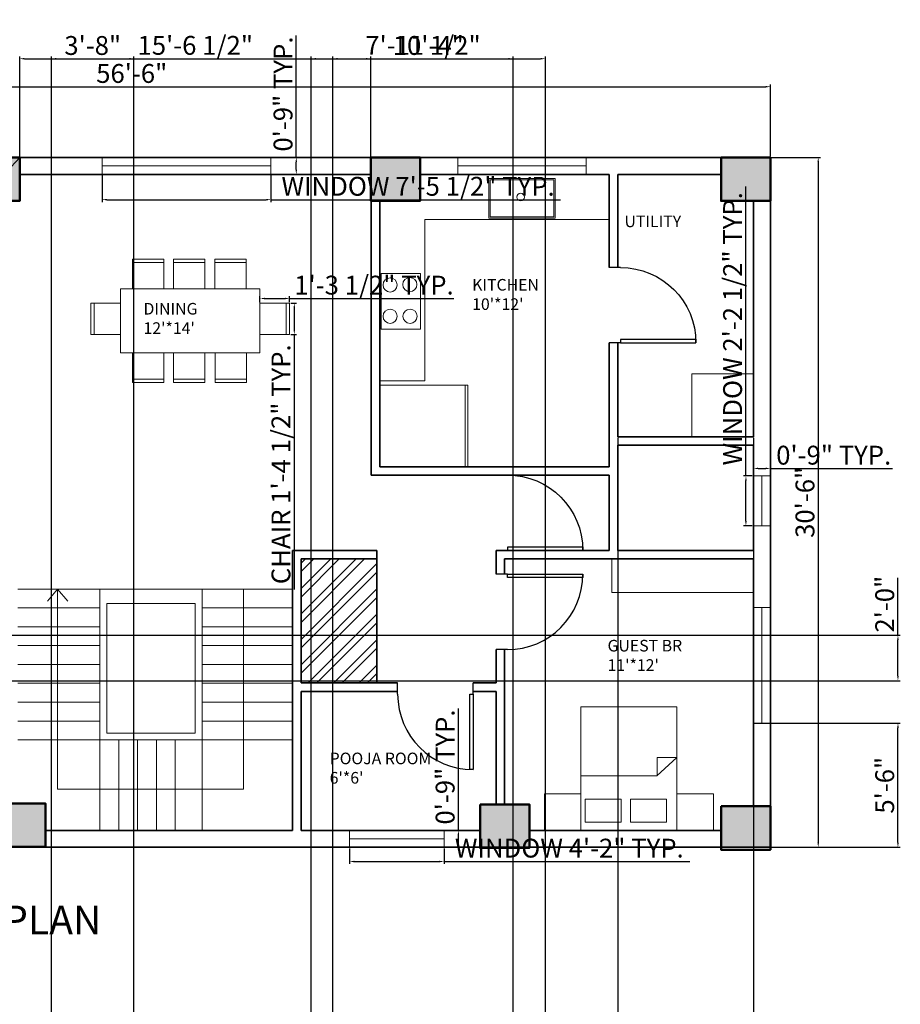
# Model space of a CAD drawing. Units: inches. Extents: x 1964 to 3462, y 1879 to 2909.
# Tile 4 of 4: x 2982 to 3450, y 2387 to 2909. Entities that reach past the tile are written whole.
import ezdxf

# ---------------------------------------------------------------- set-up
doc = ezdxf.new("R2010")
doc.units = ezdxf.units.IN
for name, color, linetype, lineweight in [('A-ANNO-DIMS', 2, 'Continuous', 18), ('A-ANNO-TEXT', 7, 'Continuous', 35), ('A-AREA-IDEN', 7, 'Continuous', 18), ('A-COLS', 1, 'Continuous', 50), ('A-COLS-PATT', 252, 'Continuous', 13), ('A-DOOR', 4, 'Continuous', 25), ('A-EQPM', 9, 'Continuous', 18), ('A-FLOR-CASE', 9, 'Continuous', 18), ('A-FLOR-FIXT', 4, 'Continuous', 18), ('A-FLOR-OPEN', 8, 'Continuous', 13), ('A-FLOR-PATT', 252, 'Continuous', 13), ('A-FLOR-STRS', 3, 'Continuous', 18), ('A-FURN', 8, 'Continuous', 18), ('A-GLAZ', 4, 'Continuous', 18), ('A-WALL', 7, 'Continuous', 35)]:
    doc.layers.add(name, color=color, linetype=linetype, lineweight=lineweight)
doc.styles.get("Standard").update_dxf_attribs({"font": 'arial.ttf'})
doc.dimstyles.new('ISO-25', dxfattribs={"dimtxt": 10, "dimasz": 2.5, "dimexe": 1.25, "dimexo": 0.625, "dimtad": 1, "dimdec": 0, "dimlunit": 4, "dimtxsty": 'Standard', "dimcen": 2.5, "dimadec": 0, "dimazin": 0, "dimtfac": 1, "dimtdec": 0, "dimtmove": 0, "dimatfit": 3, "dimfxl": 1, "dimarcsym": 0})

# ---------------------------------------------------------------- blocks, each defined once
blk = doc.blocks.new('*U2')
for p, q in [((0, 0), (0, -6)), ((40, 0), (40, -6))]:
    blk.add_line(p, q)
blk.add_lwpolyline([(0, 0), (0, 40), (1.75, 40), (1.75, 0)], close=True)
blk.add_arc((0, 0), 40, 0, 90)
blk = doc.blocks.new('*D9')
at = {"layer": 'A-ANNO-DIMS', "color": 0, "lineweight": -2, "transparency": 16777216}
for p, q in [((2702.98, 2836.98), (2702.98, 2875.1)), ((2705.48, 2873.85), (3378.17, 2873.85)), ((3380.67, 2836.98), (3380.67, 2875.1))]:
    blk.add_line(p, q, dxfattribs=at)
at = {"layer": 'A-ANNO-DIMS', "color": 0, "lineweight": 100, "transparency": 16777216}
for points in [[(2705.48, 2874.26), (2705.48, 2873.43), (2702.98, 2873.85)], [(3378.17, 2874.26), (3378.17, 2873.43), (3380.67, 2873.85)]]:
    blk.add_solid(points, dxfattribs=at)
at = {"layer": 'Defpoints', "color": 0, "lineweight": 100, "transparency": 16777216}
for p in [(3380.67, 2873.85), (2702.98, 2836.36), (3380.67, 2836.36)]:
    blk.add_point(p, dxfattribs=at)
at = {"layer": 'A-ANNO-DIMS', "color": 0, "transparency": 16777216, "insert": (3041.82, 2879.58), "char_height": 10, "attachment_point": 5}
blk.add_mtext('56\'-6"', dxfattribs=at)
blk = doc.blocks.new('*D10')
at = {"layer": 'A-ANNO-DIMS', "color": 0, "lineweight": -2, "transparency": 16777216}
for p, q in [((3381.3, 2836.36), (3407.29, 2836.36)), ((3406.04, 2833.86), (3406.04, 2472.86)), ((3381.3, 2470.36), (3407.29, 2470.36))]:
    blk.add_line(p, q, dxfattribs=at)
at = {"layer": 'A-ANNO-DIMS', "color": 0, "lineweight": 100, "transparency": 16777216}
for points in [[(3405.63, 2833.86), (3406.46, 2833.86), (3406.04, 2836.36)], [(3405.63, 2472.86), (3406.46, 2472.86), (3406.04, 2470.36)]]:
    blk.add_solid(points, dxfattribs=at)
at = {"layer": 'Defpoints', "color": 0, "lineweight": 100, "transparency": 16777216}
for p in [(3380.67, 2836.36), (3380.67, 2470.36), (3406.04, 2470.36)]:
    blk.add_point(p, dxfattribs=at)
at = {"layer": 'A-ANNO-DIMS', "color": 0, "transparency": 16777216, "insert": (3400.31, 2653.36), "char_height": 10, "attachment_point": 5, "rotation": 90}
blk.add_mtext('30\'-6"', dxfattribs=at)
blk = doc.blocks.new('COL-RECT-26x23')
blk.add_lwpolyline([(0, 23.08), (26.15, 23.08), (26.15, 0), (0, 0)], close=True)
blk = doc.blocks.new('BED-DOUBLE-WITH-NIGHTSTANDS')
for p, q in [((59.67, 28.98), (70.38, 38.71)), ((70.38, 38.71), (59.8, 38.58)), ((59.8, 38.58), (59.8, 29.09)), ((19.34, 28.98), (59.67, 28.98))]:
    blk.add_line(p, q)
for points in [[(19.34, 0), (70.38, 0), (70.38, 65.5), (19.34, 65.5)], [(19.34, 0), (0, 0), (0, 19.34), (19.34, 19.34)], [(21.67, 4.3), (40.69, 4.3), (40.69, 16.59), (21.67, 16.59)], [(45.74, 4.3), (64.76, 4.3), (64.76, 16.59), (45.74, 16.59)], [(89.72, 0), (70.38, 0), (70.38, 19.34), (89.72, 19.34)]]:
    blk.add_lwpolyline(points, close=True)
blk = doc.blocks.new('CHAIR-DINING')
blk.add_line((0, 13.93), (16.58, 13.93))
blk.add_lwpolyline([(0, 0), (16.58, 0), (16.58, 15.73), (0, 15.73)], close=True)
blk = doc.blocks.new('STAIR-RETURN-RESIDENTIAL')
for p, q in [((0, 128), (145.76, 128)), ((21.08, 128), (15.66, 121.5)), ((21.08, 21.87), (21.08, 128)), ((21.08, 128), (26.5, 121.5)), ((43.5, 124.05), (43.5, 128)), ((97.76, 128), (97.76, 118)), ((119.78, 128), (119.78, 21.87)), ((43.5, 48), (43.5, 124.05)), ((47.14, 51.64), (47.14, 120.41)), ((47.14, 120.41), (94.12, 120.41)), ((94.12, 51.64), (94.12, 120.41)), ((97.76, 48), (97.76, 124.05)), ((0, 118), (43.5, 118)), ((97.76, 118), (145.76, 118)), ((0, 108), (43.5, 108)), ((97.76, 108), (145.76, 108)), ((0, 98), (43.5, 98)), ((97.76, 98), (145.76, 98)), ((0, 88), (43.5, 88)), ((97.76, 88), (145.76, 88)), ((0, 78), (43.5, 78)), ((97.76, 78), (145.76, 78)), ((0, 68), (43.5, 68)), ((97.76, 68), (145.76, 68)), ((0, 58), (43.5, 58)), ((97.76, 58), (145.76, 58)), ((0, 48), (145.76, 48)), ((97.76, 48), (43.5, 48)), ((43.5, 48), (43.5, 0)), ((94.12, 51.64), (47.14, 51.64)), ((53.5, 48), (53.5, 0)), ((63.5, 48), (63.5, 0)), ((73.5, 48), (73.5, 0)), ((83.5, 48), (83.5, 0)), ((97.76, 50.18), (97.76, 0)), ((119.78, 21.87), (21.08, 21.87))]:
    blk.add_line(p, q)
blk = doc.blocks.new('WIN-50IN')
blk.add_line((0, 4.5), (50.22, 4.5))
blk.add_lwpolyline([(0, 9), (50.22, 9), (50.22, 0), (0, 0)], close=True)
blk = doc.blocks.new('WIN-61IN')
blk.add_line((4.5, 61.35), (4.5, 0))
blk.add_lwpolyline([(0, 61.35), (9, 61.35), (9, 0), (0, 0)], close=True)
blk = doc.blocks.new('WIN-27IN')
blk.add_line((4.5, 26.51), (4.5, 0))
blk.add_lwpolyline([(0, 0), (9, 0), (9, 26.51), (0, 26.51)], close=True)
blk = doc.blocks.new('WIN-90IN')
blk.add_line((0, 4.5), (89.57, 4.5))
blk.add_lwpolyline([(0, 9), (89.57, 9), (89.57, 0), (0, 0)], close=True)
blk = doc.blocks.new('*D27')
at = {"layer": 'A-ANNO-DIMS', "color": 0, "lineweight": -2, "transparency": 16777216}
for p, q in [((3126.2, 2759.01), (3129.32, 2759.01)), ((3128.07, 2756.51), (3128.07, 2744.93)), ((3126.2, 2742.43), (3129.32, 2742.43)), ((3128.07, 2742.43), (3128.07, 2607.19))]:
    blk.add_line(p, q, dxfattribs=at)
at = {"layer": 'A-ANNO-DIMS', "color": 0, "lineweight": 100, "transparency": 16777216}
for points in [[(3127.65, 2756.51), (3128.48, 2756.51), (3128.07, 2759.01)], [(3127.65, 2744.93), (3128.48, 2744.93), (3128.07, 2742.43)]]:
    blk.add_solid(points, dxfattribs=at)
at = {"layer": 'Defpoints', "color": 0, "lineweight": 100, "transparency": 16777216}
for p in [(3125.58, 2759.01), (3125.58, 2742.43), (3128.07, 2742.43)]:
    blk.add_point(p, dxfattribs=at)
at = {"layer": 'A-ANNO-DIMS', "color": 0, "transparency": 16777216, "insert": (3122.27, 2673.56), "char_height": 10, "attachment_point": 5, "rotation": 90}
blk.add_mtext('CHAIR 1\'-4 1/2" TYP.', dxfattribs=at)
blk = doc.blocks.new('*D28')
at = {"layer": 'A-ANNO-DIMS', "color": 0, "lineweight": -2, "transparency": 16777216}
for p, q in [((3109.85, 2759.63), (3109.85, 2762.74)), ((3112.35, 2761.49), (3123.08, 2761.49)), ((3125.58, 2759.63), (3125.58, 2762.74)), ((3125.58, 2761.49), (3212.64, 2761.49))]:
    blk.add_line(p, q, dxfattribs=at)
at = {"layer": 'A-ANNO-DIMS', "color": 0, "lineweight": 100, "transparency": 16777216}
for points in [[(3112.35, 2761.91), (3112.35, 2761.08), (3109.85, 2761.49)], [(3123.08, 2761.91), (3123.08, 2761.08), (3125.58, 2761.49)]]:
    blk.add_solid(points, dxfattribs=at)
at = {"layer": 'Defpoints', "color": 0, "lineweight": 100, "transparency": 16777216}
for p in [(3109.85, 2759.01), (3125.58, 2761.49), (3125.58, 2759.01)]:
    blk.add_point(p, dxfattribs=at)
at = {"layer": 'A-ANNO-DIMS', "color": 0, "transparency": 16777216, "insert": (3170.36, 2767.29), "char_height": 10, "attachment_point": 5}
blk.add_mtext('1\'-3 1/2" TYP.', dxfattribs=at)
blk = doc.blocks.new('*D35')
at = {"layer": 'A-ANNO-DIMS', "color": 0, "lineweight": -2, "transparency": 16777216}
for p, q in [((3157.37, 2469.73), (3157.37, 2461.58)), ((3207.59, 2469.73), (3207.59, 2461.58)), ((3159.87, 2462.83), (3205.09, 2462.83)), ((3207.59, 2462.83), (3337.88, 2462.83))]:
    blk.add_line(p, q, dxfattribs=at)
at = {"layer": 'A-ANNO-DIMS', "color": 0, "lineweight": 100, "transparency": 16777216}
for points in [[(3159.87, 2463.24), (3159.87, 2462.41), (3157.37, 2462.83)], [(3205.09, 2463.24), (3205.09, 2462.41), (3207.59, 2462.83)]]:
    blk.add_solid(points, dxfattribs=at)
at = {"layer": 'Defpoints', "color": 0, "lineweight": 100, "transparency": 16777216}
for p in [(3157.37, 2470.36), (3207.59, 2470.36), (3207.59, 2462.83)]:
    blk.add_point(p, dxfattribs=at)
at = {"layer": 'A-ANNO-DIMS', "color": 0, "transparency": 16777216, "insert": (3273.98, 2468.63), "char_height": 10, "attachment_point": 5}
blk.add_mtext('WINDOW 4\'-2" TYP.', dxfattribs=at)
blk = doc.blocks.new('*D36')
at = {"layer": 'A-ANNO-DIMS', "color": 0, "lineweight": -2, "transparency": 16777216}
for p, q in [((3215.12, 2479.36), (3215.12, 2544.06)), ((3208.21, 2479.36), (3216.37, 2479.36)), ((3215.12, 2472.86), (3215.12, 2476.86)), ((3208.21, 2470.36), (3216.37, 2470.36))]:
    blk.add_line(p, q, dxfattribs=at)
at = {"layer": 'A-ANNO-DIMS', "color": 0, "lineweight": 100, "transparency": 16777216}
for points in [[(3214.7, 2476.86), (3215.54, 2476.86), (3215.12, 2479.36)], [(3214.7, 2472.86), (3215.54, 2472.86), (3215.12, 2470.36)]]:
    blk.add_solid(points, dxfattribs=at)
at = {"layer": 'Defpoints', "color": 0, "lineweight": 100, "transparency": 16777216}
for p in [(3207.59, 2479.36), (3215.12, 2479.36), (3207.59, 2470.36)]:
    blk.add_point(p, dxfattribs=at)
at = {"layer": 'A-ANNO-DIMS', "color": 0, "transparency": 16777216, "insert": (3209.39, 2512.96), "char_height": 10, "attachment_point": 5, "rotation": 90}
blk.add_mtext('0\'-9" TYP.', dxfattribs=at)
blk = doc.blocks.new('*D39')
at = {"layer": 'A-ANNO-DIMS', "color": 0, "lineweight": -2, "transparency": 16777216}
for p, q in [((3367.7, 2667.38), (3367.7, 2820.98)), ((3371.05, 2667.38), (3366.45, 2667.38)), ((3367.7, 2643.38), (3367.7, 2664.88)), ((3371.05, 2640.88), (3366.45, 2640.88))]:
    blk.add_line(p, q, dxfattribs=at)
at = {"layer": 'A-ANNO-DIMS', "color": 0, "lineweight": 100, "transparency": 16777216}
for points in [[(3367.28, 2664.88), (3368.11, 2664.88), (3367.7, 2667.38)], [(3367.28, 2643.38), (3368.11, 2643.38), (3367.7, 2640.88)]]:
    blk.add_solid(points, dxfattribs=at)
at = {"layer": 'Defpoints', "color": 0, "lineweight": 100, "transparency": 16777216}
for p in [(3367.7, 2667.38), (3371.67, 2667.38), (3371.67, 2640.88)]:
    blk.add_point(p, dxfattribs=at)
at = {"layer": 'A-ANNO-DIMS', "color": 0, "transparency": 16777216, "insert": (3361.9, 2745.43), "char_height": 10, "attachment_point": 5, "rotation": 90}
blk.add_mtext('WINDOW 2\'-2 1/2" TYP.', dxfattribs=at)
blk = doc.blocks.new('*D40')
at = {"layer": 'A-ANNO-DIMS', "color": 0, "lineweight": -2, "transparency": 16777216}
for p, q in [((3371.67, 2668.01), (3371.67, 2672.61)), ((3374.17, 2671.36), (3378.17, 2671.36)), ((3380.67, 2668.01), (3380.67, 2672.61)), ((3380.67, 2671.36), (3445.38, 2671.36))]:
    blk.add_line(p, q, dxfattribs=at)
at = {"layer": 'A-ANNO-DIMS', "color": 0, "lineweight": 100, "transparency": 16777216}
for points in [[(3374.17, 2671.78), (3374.17, 2670.94), (3371.67, 2671.36)], [(3378.17, 2671.78), (3378.17, 2670.94), (3380.67, 2671.36)]]:
    blk.add_solid(points, dxfattribs=at)
at = {"layer": 'Defpoints', "color": 0, "lineweight": 100, "transparency": 16777216}
for p in [(3380.67, 2671.36), (3371.67, 2667.38), (3380.67, 2667.38)]:
    blk.add_point(p, dxfattribs=at)
at = {"layer": 'A-ANNO-DIMS', "color": 0, "transparency": 16777216, "insert": (3414.27, 2677.09), "char_height": 10, "attachment_point": 5}
blk.add_mtext('0\'-9" TYP.', dxfattribs=at)
blk = doc.blocks.new('*D41')
at = {"layer": 'A-ANNO-DIMS', "color": 0, "lineweight": -2, "transparency": 16777216}
for p, q in [((3026.12, 2826.73), (3026.12, 2812.67)), ((3115.69, 2826.73), (3115.69, 2812.67)), ((3028.62, 2813.92), (3113.19, 2813.92)), ((3115.69, 2813.92), (3269.28, 2813.92))]:
    blk.add_line(p, q, dxfattribs=at)
at = {"layer": 'A-ANNO-DIMS', "color": 0, "lineweight": 100, "transparency": 16777216}
for points in [[(3028.62, 2814.34), (3028.62, 2813.51), (3026.12, 2813.92)], [(3113.19, 2814.34), (3113.19, 2813.51), (3115.69, 2813.92)]]:
    blk.add_solid(points, dxfattribs=at)
at = {"layer": 'Defpoints', "color": 0, "lineweight": 100, "transparency": 16777216}
for p in [(3026.12, 2827.36), (3115.69, 2827.36), (3115.69, 2813.92)]:
    blk.add_point(p, dxfattribs=at)
at = {"layer": 'A-ANNO-DIMS', "color": 0, "transparency": 16777216, "insert": (3193.74, 2819.72), "char_height": 10, "attachment_point": 5}
blk.add_mtext('WINDOW 7\'-5 1/2" TYP.', dxfattribs=at)
blk = doc.blocks.new('*D42')
at = {"layer": 'A-ANNO-DIMS', "color": 0, "lineweight": -2, "transparency": 16777216}
for p, q in [((3129.13, 2836.36), (3129.13, 2901.06)), ((3116.32, 2836.36), (3130.38, 2836.36)), ((3129.13, 2829.86), (3129.13, 2833.86)), ((3116.32, 2827.36), (3130.38, 2827.36))]:
    blk.add_line(p, q, dxfattribs=at)
at = {"layer": 'A-ANNO-DIMS', "color": 0, "lineweight": 100, "transparency": 16777216}
for points in [[(3128.71, 2833.86), (3129.54, 2833.86), (3129.13, 2836.36)], [(3128.71, 2829.86), (3129.54, 2829.86), (3129.13, 2827.36)]]:
    blk.add_solid(points, dxfattribs=at)
at = {"layer": 'Defpoints', "color": 0, "lineweight": 100, "transparency": 16777216}
for p in [(3115.69, 2836.36), (3129.13, 2836.36), (3115.69, 2827.36)]:
    blk.add_point(p, dxfattribs=at)
at = {"layer": 'A-ANNO-DIMS', "color": 0, "transparency": 16777216, "insert": (3123.39, 2869.96), "char_height": 10, "attachment_point": 5, "rotation": 90}
blk.add_mtext('0\'-9" TYP.', dxfattribs=at)
blk = doc.blocks.new('*D55')
at = {"layer": 'A-ANNO-DIMS', "color": 0, "lineweight": -2, "transparency": 16777216}
for p, q in [((2982.37, 2813.9), (2982.37, 2889.94)), ((2984.87, 2888.69), (3166.19, 2888.69)), ((3168.69, 2813.9), (3168.69, 2889.94))]:
    blk.add_line(p, q, dxfattribs=at)
at = {"layer": 'A-ANNO-DIMS', "color": 0, "lineweight": 100, "transparency": 16777216}
for points in [[(2984.87, 2889.1), (2984.87, 2888.27), (2982.37, 2888.69)], [(3166.19, 2889.1), (3166.19, 2888.27), (3168.69, 2888.69)]]:
    blk.add_solid(points, dxfattribs=at)
at = {"layer": 'Defpoints', "color": 0, "lineweight": 100, "transparency": 16777216}
for p in [(3168.69, 2888.69), (2982.37, 2813.28), (3168.69, 2813.28)]:
    blk.add_point(p, dxfattribs=at)
at = {"layer": 'A-ANNO-DIMS', "color": 0, "transparency": 16777216, "insert": (3075.53, 2894.48), "char_height": 10, "attachment_point": 5}
blk.add_mtext('15\'-6 1/2"', dxfattribs=at)
blk = doc.blocks.new('*D56')
at = {"layer": 'A-ANNO-DIMS', "color": 0, "lineweight": -2, "transparency": 16777216}
for p, q in [((3299.67, 2687.56), (3299.67, 1887.22)), ((3371.67, 2687.56), (3371.67, 1887.22)), ((3302.17, 1888.47), (3369.17, 1888.47))]:
    blk.add_line(p, q, dxfattribs=at)
at = {"layer": 'A-ANNO-DIMS', "color": 0, "lineweight": 100, "transparency": 16777216}
for points in [[(3302.17, 1888.89), (3302.17, 1888.06), (3299.67, 1888.47)], [(3369.17, 1888.89), (3369.17, 1888.06), (3371.67, 1888.47)]]:
    blk.add_solid(points, dxfattribs=at)
at = {"layer": 'Defpoints', "color": 0, "lineweight": 100, "transparency": 16777216}
for p in [(3299.67, 2688.18), (3371.67, 2688.18), (3371.67, 1888.47)]:
    blk.add_point(p, dxfattribs=at)
at = {"layer": 'A-ANNO-DIMS', "color": 0, "transparency": 16777216, "insert": (3335.67, 1894.2), "char_height": 10, "attachment_point": 5}
blk.add_mtext('6\'-0"', dxfattribs=at)
blk = doc.blocks.new('*D60')
at = {"layer": 'A-ANNO-DIMS', "color": 0, "lineweight": -2, "transparency": 16777216}
for p, q in [((3448.35, 2582.86), (3448.35, 2613.36)), ((2815.81, 2582.86), (3449.6, 2582.86)), ((3448.35, 2561.25), (3448.35, 2580.36)), ((2815.81, 2558.75), (3449.6, 2558.75))]:
    blk.add_line(p, q, dxfattribs=at)
at = {"layer": 'A-ANNO-DIMS', "color": 0, "lineweight": 100, "transparency": 16777216}
for points in [[(3447.94, 2580.36), (3448.77, 2580.36), (3448.35, 2582.86)], [(3447.94, 2561.25), (3448.77, 2561.25), (3448.35, 2558.75)]]:
    blk.add_solid(points, dxfattribs=at)
at = {"layer": 'Defpoints', "color": 0, "lineweight": 100, "transparency": 16777216}
for p in [(2815.18, 2582.86), (3448.35, 2582.86), (2815.18, 2558.75)]:
    blk.add_point(p, dxfattribs=at)
at = {"layer": 'A-ANNO-DIMS', "color": 0, "transparency": 16777216, "insert": (3442.62, 2599.36), "char_height": 10, "attachment_point": 5, "rotation": 90}
blk.add_mtext('2\'-0"', dxfattribs=at)
blk = doc.blocks.new('*D61')
at = {"layer": 'A-ANNO-DIMS', "color": 0, "lineweight": -2, "transparency": 16777216}
for p, q in [((3372.3, 2536.22), (3449.6, 2536.22)), ((3448.35, 2472.86), (3448.35, 2533.72)), ((3381.3, 2470.36), (3449.6, 2470.36))]:
    blk.add_line(p, q, dxfattribs=at)
at = {"layer": 'A-ANNO-DIMS', "color": 0, "lineweight": 100, "transparency": 16777216}
for points in [[(3447.94, 2533.72), (3448.77, 2533.72), (3448.35, 2536.22)], [(3447.94, 2472.86), (3448.77, 2472.86), (3448.35, 2470.36)]]:
    blk.add_solid(points, dxfattribs=at)
at = {"layer": 'Defpoints', "color": 0, "lineweight": 100, "transparency": 16777216}
for p in [(3371.67, 2536.22), (3448.35, 2536.22), (3380.67, 2470.36)]:
    blk.add_point(p, dxfattribs=at)
at = {"layer": 'A-ANNO-DIMS', "color": 0, "transparency": 16777216, "insert": (3442.62, 2503.29), "char_height": 10, "attachment_point": 5, "rotation": 90}
blk.add_mtext('5\'-6"', dxfattribs=at)
blk = doc.blocks.new('*D65')
at = {"layer": 'A-ANNO-DIMS', "color": 0, "lineweight": -2, "transparency": 16777216}
for p, q in [((3137.07, 2298.2), (3137.07, 2889.94)), ((3139.57, 2888.69), (3258.77, 2888.69)), ((3261.27, 2298.2), (3261.27, 2889.94))]:
    blk.add_line(p, q, dxfattribs=at)
at = {"layer": 'A-ANNO-DIMS', "color": 0, "lineweight": 100, "transparency": 16777216}
for points in [[(3139.57, 2889.1), (3139.57, 2888.27), (3137.07, 2888.69)], [(3258.77, 2889.1), (3258.77, 2888.27), (3261.27, 2888.69)]]:
    blk.add_solid(points, dxfattribs=at)
at = {"layer": 'Defpoints', "color": 0, "lineweight": 100, "transparency": 16777216}
for p in [(3261.27, 2888.69), (3137.07, 2297.57), (3261.27, 2297.57)]:
    blk.add_point(p, dxfattribs=at)
at = {"layer": 'A-ANNO-DIMS', "color": 0, "transparency": 16777216, "insert": (3199.17, 2894.42), "char_height": 10, "attachment_point": 5}
blk.add_mtext('10\'-4"', dxfattribs=at)
blk = doc.blocks.new('*D67')
at = {"layer": 'A-ANNO-DIMS', "color": 0, "lineweight": -2, "transparency": 16777216}
for p, q in [((3148.55, 2033.75), (3148.55, 2889.94)), ((3151.05, 2888.69), (3241.63, 2888.69)), ((3244.13, 2034), (3244.13, 2889.94))]:
    blk.add_line(p, q, dxfattribs=at)
at = {"layer": 'A-ANNO-DIMS', "color": 0, "lineweight": 100, "transparency": 16777216}
for points in [[(3151.05, 2889.1), (3151.05, 2888.27), (3148.55, 2888.69)], [(3241.63, 2889.1), (3241.63, 2888.27), (3244.13, 2888.69)]]:
    blk.add_solid(points, dxfattribs=at)
at = {"layer": 'Defpoints', "color": 0, "lineweight": 100, "transparency": 16777216}
for p in [(3244.13, 2888.69), (3148.55, 2033.12), (3244.13, 2033.37)]:
    blk.add_point(p, dxfattribs=at)
at = {"layer": 'A-ANNO-DIMS', "color": 0, "transparency": 16777216, "insert": (3196.34, 2894.48), "char_height": 10, "attachment_point": 5}
blk.add_mtext('7\'-11 1/2"', dxfattribs=at)
blk = doc.blocks.new('*D68')
at = {"layer": 'A-ANNO-DIMS', "color": 0, "lineweight": -2, "transparency": 16777216}
for p, q in [((2999.25, 2307.2), (2999.25, 2889.94)), ((3001.75, 2888.69), (3040.51, 2888.69)), ((3043.01, 2307.2), (3043.01, 2889.94))]:
    blk.add_line(p, q, dxfattribs=at)
at = {"layer": 'A-ANNO-DIMS', "color": 0, "lineweight": 100, "transparency": 16777216}
for points in [[(3001.75, 2889.1), (3001.75, 2888.27), (2999.25, 2888.69)], [(3040.51, 2889.1), (3040.51, 2888.27), (3043.01, 2888.69)]]:
    blk.add_solid(points, dxfattribs=at)
at = {"layer": 'Defpoints', "color": 0, "lineweight": 100, "transparency": 16777216}
for p in [(3043.01, 2888.69), (2999.25, 2306.57), (3043.01, 2306.57)]:
    blk.add_point(p, dxfattribs=at)
at = {"layer": 'A-ANNO-DIMS', "color": 0, "transparency": 16777216, "insert": (3021.13, 2894.42), "char_height": 10, "attachment_point": 5}
blk.add_mtext('3\'-8"', dxfattribs=at)

msp = doc.modelspace()

# ---------------------------------------------------------------- hatches: boundary and pattern name
at = {"layer": 'A-COLS-PATT'}
h = msp.add_hatch(color=256, dxfattribs=at)
h.dxf.hatch_style = 1
h.paths.add_polyline_path([(3380.67, 2836.36), (3354.52, 2836.36), (3354.52, 2813.28), (3380.67, 2813.28)])
h.paths.add_polyline_path([(3194.85, 2836.36), (3168.69, 2836.36), (3168.69, 2827.36), (3168.91, 2827.36), (3168.91, 2813.28), (3194.85, 2813.28)])
h.paths.add_polyline_path([(2982.37, 2836.36), (2956.21, 2836.36), (2956.21, 2813.28), (2961, 2813.28)])
h.paths.add_polyline_path([(2982.37, 2836.36), (2961, 2813.28), (2981.41, 2813.28), (2982.37, 2813.28)], flags=17)
h.paths.add_polyline_path([(2831.78, 2494.67), (2805.62, 2494.67), (2805.62, 2471.58), (2831.78, 2471.58)])
h.paths.add_polyline_path([(2995.98, 2493.63), (2969.83, 2493.63), (2969.83, 2470.55), (2995.98, 2470.55)])
h.paths.add_polyline_path([(3252.83, 2493.16), (3226.67, 2493.16), (3226.67, 2470.36), (3252.83, 2470.36)])
h.paths.add_polyline_path([(3380.67, 2492.15), (3354.52, 2492.15), (3354.52, 2470.36), (3380.67, 2470.36)])
at = {"layer": 'A-FLOR-PATT'}
h = msp.add_hatch(dxfattribs=at)
h.set_pattern_fill('ANSI32', color=256)
h.set_pattern_definition([(45, (161.698, 257.281), (-6.735192, 6.735192), []), (45, (166.188, 257.281), (-6.735192, 6.735192), [])])
h.paths.add_polyline_path([(3131.67, 2557.57), (3171.89, 2557.57), (3171.89, 2623.36), (3131.67, 2623.36)])
h.paths.add_polyline_path([(3164.38, 2278.1), (3261.27, 2278.1), (3261.27, 2297.57), (3231.68, 2297.57), (3211.73, 2297.57), (3211.73, 2283.49), (3185.58, 2283.49), (3185.58, 2297.57), (3166.29, 2297.57), (3142.29, 2297.57), (3137.07, 2297.57), (3137.07, 2154.78), (3164.38, 2154.78)])
h.paths.add_polyline_path([(2977.34, 2283.49), (2973.1, 2283.49), (2973.1, 2297.57), (2946.77, 2297.57), (2946.77, 2213.49), (2977.34, 2213.49)])
h.paths.add_polyline_path([(3313.48, 2093.57), (3313.48, 2075.7), (3388.55, 2075.7), (3388.55, 2093.57)])
h.paths.add_polyline_path([(3161.01, 2228.59), (3238.21, 2228.59), (3238.21, 2241.28), (3161.01, 2241.28)], flags=24)

# ---------------------------------------------------------------- linework, layer by layer
at = {"layer": 'A-EQPM'}
for points in [[(3174.19, 2774.84), (3195.11, 2774.84), (3195.11, 2745.16), (3174.19, 2745.16)], [(3371.67, 2688.18), (3339, 2688.18), (3339, 2721.57), (3371.67, 2721.57)]]:
    msp.add_lwpolyline(points, close=True, dxfattribs=at)
for centre in [(3178.9, 2768.68), (3189.36, 2768.89), (3178.9, 2752.06), (3189.47, 2752.06)]:
    msp.add_circle(centre, 3.76, dxfattribs=at)
at = {"layer": 'A-FLOR-CASE'}
for p, q in [((3295.17, 2827.36), (3295.17, 2803.36)), ((3197.41, 2717.82), (3197.41, 2803.36)), ((3295.17, 2803.36), (3197.41, 2803.36)), ((3173.41, 2717.82), (3197.41, 2717.82)), ((3218.8, 2672.28), (3218.8, 2715.58))]:
    msp.add_line(p, q, dxfattribs=at)
for points in [[(3173.41, 2672.28), (3220.22, 2672.28), (3220.22, 2715.58), (3173.41, 2715.58)], [(3371.67, 2623.36), (3296.59, 2623.36), (3296.59, 2605.49), (3371.67, 2605.49)]]:
    msp.add_lwpolyline(points, close=True, dxfattribs=at)
at = {"layer": 'A-FLOR-FIXT'}
for points in [[(3231.34, 2804.15), (3266.43, 2804.15), (3266.43, 2825.23), (3231.34, 2825.23)], [(3232.07, 2804.88), (3265.7, 2804.88), (3265.7, 2824.5), (3232.07, 2824.5)]]:
    msp.add_lwpolyline(points, close=True, dxfattribs=at)
msp.add_circle((3248.15, 2815.32), 1.98, dxfattribs=at)
at = {"layer": 'A-FLOR-OPEN'}
msp.add_line((2751.91, 2587.36), (2982.37, 2836.36), dxfattribs=at)
at = {"layer": 'A-FLOR-STRS'}
for q in [(3127.17, 2515.36), (3091.17, 2479.36), (3091.17, 2479.36)]:
    msp.add_line((3127.17, 2479.36), q, dxfattribs=at)
at = {"layer": 'A-FURN'}
msp.add_lwpolyline([(3035.8, 2766.67), (3109.85, 2766.67), (3109.85, 2732.61), (3035.8, 2732.61)], close=True, dxfattribs=at)
at = {"layer": 'A-GLAZ'}
msp.add_line((3214.8, 2831.86), (3282.98, 2831.86), dxfattribs=at)
msp.add_lwpolyline([(3214.8, 2836.36), (3282.98, 2836.36), (3282.98, 2827.36), (3214.8, 2827.36)], close=True, dxfattribs=at)
at = {"layer": 'A-WALL'}
for p, q in [((3380.67, 2836.36), (3380.67, 2470.36)), ((2982.37, 2827.36), (3125.41, 2827.36)), ((3125.41, 2827.36), (3149.41, 2827.36)), ((3149.41, 2827.36), (3168.91, 2827.36)), ((3168.91, 2827.36), (3168.91, 2667.78)), ((3295.17, 2827.36), (3295.17, 2777.95)), ((3354.52, 2827.36), (3299.67, 2827.36)), ((3299.67, 2827.36), (3299.67, 2777.95)), ((3173.41, 2813.28), (3173.41, 2672.28)), ((3295.17, 2737.95), (3295.17, 2707.36)), ((3299.67, 2737.95), (3299.67, 2707.36)), ((3295.17, 2707.36), (3295.17, 2672.28)), ((3299.67, 2707.36), (3299.67, 2688.18)), ((3299.67, 2688.18), (3371.67, 2688.18)), ((3299.67, 2683.68), (3371.67, 2683.68)), ((3299.67, 2683.68), (3299.67, 2627.86)), ((3355.57, 2683.68), (3371.67, 2683.68)), ((3295.17, 2672.28), (3173.41, 2672.28)), ((3295.17, 2667.78), (3168.91, 2667.78)), ((3295.17, 2667.78), (3295.17, 2627.86)), ((3127.17, 2479.36), (3127.17, 2627.86)), ((3127.17, 2627.86), (3171.89, 2627.86)), ((3171.89, 2557.57), (3171.89, 2627.86)), ((3235.17, 2623.36), (3235.17, 2627.86)), ((3235.17, 2627.86), (3246.85, 2627.86)), ((3295.17, 2627.86), (3235.17, 2627.86)), ((3371.67, 2627.86), (3299.67, 2627.86)), ((3131.67, 2623.36), (3171.89, 2623.36)), ((3131.67, 2557.57), (3131.67, 2623.36)), ((3235.17, 2623.36), (3235.17, 2615.22)), ((3371.67, 2623.36), (3239.67, 2623.36)), ((3239.67, 2623.36), (3239.67, 2615.22)), ((3239.67, 2623.36), (3246.85, 2623.36)), ((3371.67, 2492.15), (3371.67, 2623.36)), ((3235.17, 2575.22), (3235.17, 2557.57)), ((3239.67, 2575.22), (3239.67, 2493.16)), ((3131.67, 2557.57), (3182.9, 2557.57)), ((3222.9, 2557.57), (3235.17, 2557.57)), ((3131.67, 2479.36), (3131.67, 2553.07)), ((3131.67, 2553.07), (3182.9, 2553.07)), ((3222.9, 2553.07), (3235.17, 2553.07)), ((3235.17, 2553.07), (3235.17, 2493.16)), ((3163.17, 2479.36), (3131.67, 2479.36)), ((3226.67, 2479.36), (3163.17, 2479.36))]:
    msp.add_line(p, q, dxfattribs=at)
for points in [[(2751.91, 2633.6), (2751.91, 2836.36), (3380.67, 2836.36), (3380.67, 2470.36), (2751.91, 2470.36)], [(3380.67, 2674.12), (3380.67, 2836.36), (2841.75, 2836.36)], [(2982.37, 2827.36), (3168.91, 2827.36)], [(3194.85, 2827.36), (3295.17, 2827.36)], [(3299.67, 2827.36), (3354.52, 2827.36)], [(3371.67, 2813.28), (3371.67, 2688.18)], [(3371.67, 2683.68), (3371.67, 2627.86)], [(2841.75, 2470.36), (3380.67, 2470.36), (3380.67, 2634.12)], [(3371.67, 2623.36), (3371.67, 2492.15)], [(3127.17, 2479.36), (2995.98, 2479.36)], [(3226.67, 2479.36), (3131.67, 2479.36)], [(3354.52, 2479.36), (3252.83, 2479.36)]]:
    msp.add_lwpolyline(points, dxfattribs=at)

# ---------------------------------------------------------------- block references
at = {"layer": 'A-COLS'}
for p in [(2956.21, 2813.28), (3168.69, 2813.28), (3354.52, 2813.28), (2969.83, 2470.55), (3226.67, 2470.08), (3354.52, 2469.06)]:
    msp.add_blockref('COL-RECT-26x23', p, dxfattribs=at)
at = {"layer": 'A-DOOR', "xscale": -1, "rotation": 270}
for p in [(3301.17, 2737.95), (3241.17, 2627.86)]:
    msp.add_blockref('*U2', p, dxfattribs=at)
at = {"layer": 'A-DOOR'}
for p, rotation in [((3241.17, 2615.22), 270), ((3222.9, 2551.57), 180)]:
    msp.add_blockref('*U2', p, dxfattribs=dict(at, rotation=rotation))
at = {"layer": 'A-FLOR-STRS'}
msp.add_blockref('STAIR-RETURN-RESIDENTIAL', (2981.41, 2479.36), dxfattribs=at)
at = {"layer": 'A-FURN'}
for name, p in [('CHAIR-DINING', (3042.19, 2766.67)), ('CHAIR-DINING', (3063.95, 2766.67)), ('CHAIR-DINING', (3085.97, 2766.67)), ('BED-DOUBLE-WITH-NIGHTSTANDS', (3260.74, 2479.36))]:
    msp.add_blockref(name, p, dxfattribs=at)
at = {"layer": 'A-FURN', "extrusion": (0, 0, -1), "zscale": -1}
for p, rotation in [((-3035.8, 2759.01), 269.9999999999971), ((-3042.3, 2732.61), 180), ((-3064.05, 2732.61), 180), ((-3086.08, 2732.61), 180)]:
    msp.add_blockref('CHAIR-DINING', p, dxfattribs=dict(at, rotation=rotation))
at = {"layer": 'A-FURN', "rotation": 269.9999999999971}
msp.add_blockref('CHAIR-DINING', (3109.85, 2759.01), dxfattribs=at)
at = {"layer": 'A-GLAZ'}
for name, p in [('WIN-90IN', (3026.12, 2827.36)), ('WIN-27IN', (3371.67, 2640.88)), ('WIN-61IN', (3371.67, 2536.22)), ('WIN-50IN', (3157.37, 2470.36))]:
    msp.add_blockref(name, p, dxfattribs=at)

# ---------------------------------------------------------------- texts
at = {"layer": 'A-ANNO-TEXT', "insert": (2708.78, 2439.45), "char_height": 15.2607, "attachment_point": 1}
msp.add_mtext_dynamic_manual_height_columns('FIRST RESIDENTIAL FLOOR PLAN', width=480.7827, gutter_width=76.3, heights=[0], dxfattribs=at)
at = {"layer": 'A-AREA-IDEN', "char_height": 6.161, "attachment_point": 1}
for s, insert in [('UTILITY', (3303.25, 2805.5)), ("KITCHEN\\P10'*12'", (3222.43, 2771.85)), ("DINING\\P12'*14'", (3048.05, 2759.14)), ("GUEST BR\\P11'*12'", (3294.27, 2580.41)), ("POOJA ROOM\\P6'*6'", (3146.84, 2520.59))]:
    msp.add_mtext_dynamic_manual_height_columns(s, width=194.1034, gutter_width=30.81, heights=[0], dxfattribs=dict(at, insert=insert))

# ---------------------------------------------------------------- dimensions: what is measured, and where the dimension line sits
at = {"layer": 'A-ANNO-DIMS'}
for base, p1, p2, override, picture, middle in [((3168.69, 2888.69), (2982.37, 2813.28), (3168.69, 2813.28), {"dimdec": 1, "dimlfac": 1, "dimrnd": 0, "dimzin": 1, "dimdsep": 46, "dimlunit": 4, "dimfrac": 2}, '*D55', (3075.53, 2894.48)), ((3244.13, 2888.69), (3148.55, 2033.12), (3244.13, 2033.37), {"dimdec": 1, "dimlfac": 1, "dimrnd": 0, "dimzin": 1, "dimdsep": 46, "dimlunit": 4, "dimfrac": 2}, '*D67', (3196.34, 2894.48)), ((3043.01, 2888.69), (2999.25, 2306.57), (3043.01, 2306.57), {"dimdec": 1, "dimlfac": 1, "dimrnd": 0, "dimzin": 1, "dimdsep": 46, "dimlunit": 4, "dimfrac": 2}, '*D68', (3021.13, 2894.42)), ((3261.27, 2888.69), (3137.07, 2297.57), (3261.27, 2297.57), {"dimdec": 1, "dimlfac": 1, "dimrnd": 0, "dimzin": 1, "dimdsep": 46, "dimlunit": 4, "dimfrac": 2}, '*D65', (3199.17, 2894.42)), ((3380.67, 2873.85), (2702.98, 2836.36), (3380.67, 2836.36), {"dimclrd": 0, "dimclre": 0, "dimclrt": 0}, '*D9', (3041.82, 2879.58)), ((3371.67, 1888.47), (3299.67, 2688.18), (3371.67, 2688.18), {"dimdec": 1, "dimlfac": 1, "dimrnd": 0, "dimzin": 1, "dimdsep": 46, "dimlunit": 4, "dimfrac": 2}, '*D56', (3335.67, 1894.2))]:
    dim = msp.add_linear_dim(base=base, p1=p1, p2=p2, dimstyle='ISO-25', override=override, dxfattribs=at)
    dim.commit()
    dim.dimension.update_dxf_attribs({"geometry": picture, "text_midpoint": middle})
for base, p1, p2, angle, text, picture, middle in [((3129.13, 2836.36), (3115.69, 2827.36), (3115.69, 2836.36), 90, '<> TYP.', '*D42', (3123.39, 2869.96)), ((3367.7, 2667.38), (3371.67, 2640.88), (3371.67, 2667.38), 90, 'WINDOW <> TYP.', '*D39', (3361.9, 2745.43)), ((3128.07, 2742.43), (3125.58, 2759.01), (3125.58, 2742.43), 270, 'CHAIR <> TYP.', '*D27', (3122.27, 2673.56)), ((3215.12, 2479.36), (3207.59, 2470.36), (3207.59, 2479.36), 90, '<> TYP.', '*D36', (3209.39, 2512.96))]:
    dim = msp.add_linear_dim(base=base, p1=p1, p2=p2, angle=angle, text=text, dimstyle='ISO-25', override={"dimdec": 1, "dimlfac": 1, "dimrnd": 0, "dimzin": 1, "dimdsep": 46, "dimlunit": 4, "dimfrac": 2}, dxfattribs=at)
    dim.commit()
    dim.dimension.update_dxf_attribs({"geometry": picture, "text_midpoint": middle})
for base, p1, p2, text, picture, middle in [((3115.69, 2813.92), (3026.12, 2827.36), (3115.69, 2827.36), 'WINDOW <> TYP.', '*D41', (3193.74, 2819.72)), ((3125.58, 2761.49), (3109.85, 2759.01), (3125.58, 2759.01), '<> TYP.', '*D28', (3170.36, 2767.29)), ((3380.67, 2671.36), (3371.67, 2667.38), (3380.67, 2667.38), '<> TYP.', '*D40', (3414.27, 2677.09)), ((3207.59, 2462.83), (3157.37, 2470.36), (3207.59, 2470.36), 'WINDOW <> TYP.', '*D35', (3273.98, 2468.63))]:
    dim = msp.add_linear_dim(base=base, p1=p1, p2=p2, text=text, dimstyle='ISO-25', override={"dimdec": 1, "dimlfac": 1, "dimrnd": 0, "dimzin": 1, "dimdsep": 46, "dimlunit": 4, "dimfrac": 2}, dxfattribs=at)
    dim.commit()
    dim.dimension.update_dxf_attribs({"geometry": picture, "text_midpoint": middle})
for base, p1, p2, override, picture, middle in [((3406.04, 2470.36), (3380.67, 2836.36), (3380.67, 2470.36), {"dimclrd": 0, "dimclre": 0, "dimclrt": 0}, '*D10', (3400.31, 2653.36)), ((3448.35, 2582.86), (2815.18, 2558.75), (2815.18, 2582.86), {"dimdec": 1, "dimlfac": 1, "dimrnd": 0, "dimzin": 1, "dimdsep": 46, "dimlunit": 4, "dimfrac": 2}, '*D60', (3442.62, 2599.36)), ((3448.35, 2536.22), (3380.67, 2470.36), (3371.67, 2536.22), {"dimdec": 1, "dimlfac": 1, "dimrnd": 0, "dimzin": 1, "dimdsep": 46, "dimlunit": 4, "dimfrac": 2}, '*D61', (3442.62, 2503.29))]:
    dim = msp.add_linear_dim(base=base, p1=p1, p2=p2, angle=90, dimstyle='ISO-25', override=override, dxfattribs=at)
    dim.commit()
    dim.dimension.update_dxf_attribs({"geometry": picture, "text_midpoint": middle})

doc.saveas('drawing.dxf')
